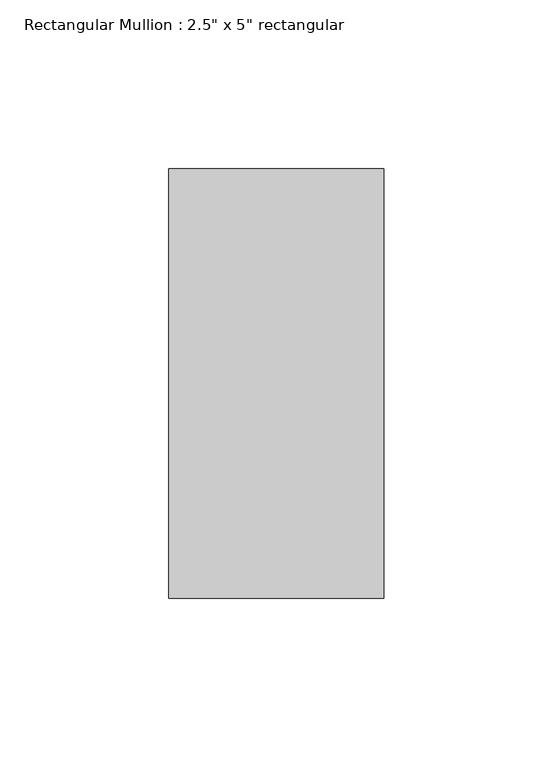
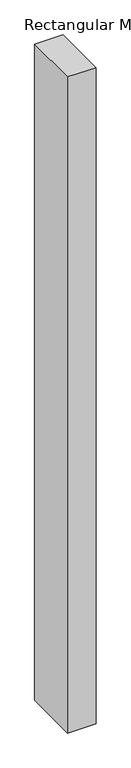
"""IFC4 building model written with IfcOpenShell, lengths in millimetres: member geometry."""

from ifc_helpers import new_model, si_unit, frame, origin, place, context, project, spatial, polyline, outline, extrude, source, transform, mapped, element, save


def member_0499d444(model_context):
    return source(origin(), model_context, "Body", "SweptSolid", [
        extrude(outline(polyline([(0.0, 63.5), (0.0, -63.5), (-63.5, -63.5), (-63.5, 63.5), (0.0, 63.5)])), frame((0.0, 0.0, -1550.242764), z_axis=(0.0, 0.0, 1.0), x_axis=(1.0, 0.0, 0.0)), (0.0, 0.0, 1.0), 1550.242764),
    ])


if __name__ == "__main__":
    model = new_model("IFC4")
    model_context = context("Model", 3, world=origin())
    ifc_project = project(units=[si_unit("LENGTHUNIT", "METRE", prefix="MILLI")], contexts=[model_context])
    site = spatial("IfcSite", under=ifc_project)
    building = spatial("IfcBuilding", under=site)
    placement = place(None, origin())
    member_shape = member_0499d444(model_context)
    element("IfcMember", 1, ObjectType="Rectangular Mullion : 2.5\" x 5\" rectangular", at=placement, inside=building, context=model_context, shape_type="MappedRepresentation", body=[
        mapped(member_shape, transform((0.0, 0.0, 0.0), x_axis=(1.0, 0.0, 0.0), y_axis=(0.0, 1.0, 0.0), z_axis=(0.0, 0.0, 1.0))),
    ])
    save(model, "model.ifc")

# Revit data of these elements
# Type "Rectangular Mullion : 2.5\" x 5\" rectangular"
#   built-in parameter 1007304 = 0.416667 (stored number, unit not read)
#   built-in parameter 1007301 = 0.104167 (stored number, unit not read)
#   built-in parameter 1007300 = 0.104167 (stored number, unit not read)
# Element 1 (IfcMember, "Rectangular Mullion : 2.5\" x 5\" rectangular")
#   Materials on its faces: "Aluminum"
# Materials
#   "Aluminum": class "Metal", colour RGB 247 247 247, transparency 0, Description = "Aluminum 6061", Cost = 0
